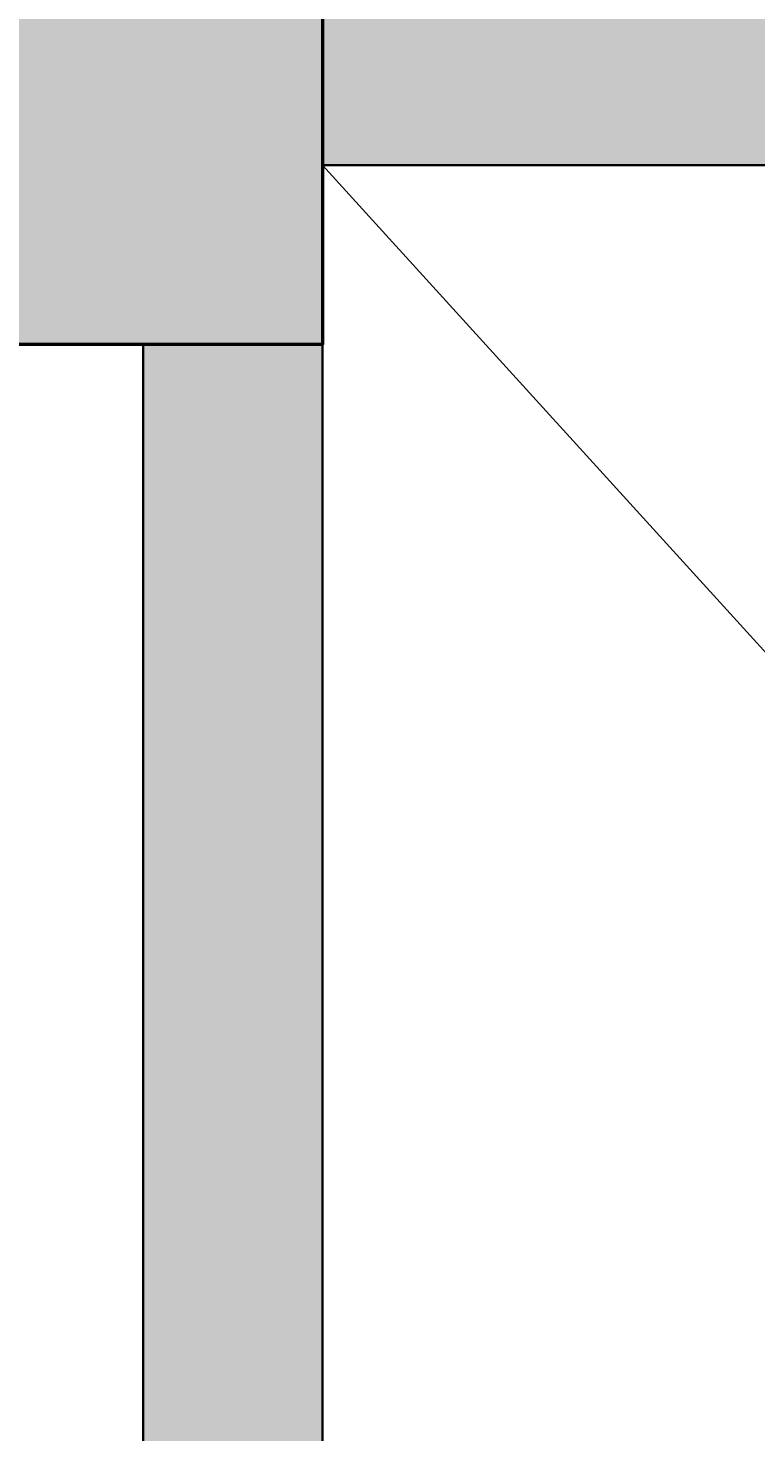
# Model space of a CAD drawing. Units: inches. Extents: x 1998 to 2588, y 1139 to 1977.
# Tile 33 of 134: x 2220 to 2238, y 1557 to 1592. Entities that reach past the tile are written whole.
import ezdxf

# ---------------------------------------------------------------- set-up
doc = ezdxf.new("R2010")
doc.units = ezdxf.units.IN
for name, color, linetype, lineweight in [('A-ANNO-DIMS', 2, 'Continuous', 18), ('A-COLS-PATT', 250, 'Continuous', 13), ('A-FLOR-OPEN', 8, 'Continuous', 18), ('A-WALL-PATT', 252, 'Continuous', 13), ('COLUMN', 10, 'Continuous', 50), ('WALL', 200, 'Continuous', 35)]:
    doc.layers.add(name, color=color, linetype=linetype, lineweight=lineweight)
doc.styles.get("Standard").update_dxf_attribs({"font": 'arial.ttf'})
doc.dimstyles.get("Standard").update_dxf_attribs({"dimtxt": 0.18, "dimasz": 0.18, "dimexe": 0.18, "dimexo": 0.0625, "dimgap": 0.09, "dimtad": 0, "dimtih": 1, "dimtoh": 1, "dimdec": 4, "dimzin": 0, "dimdsep": 46, "dimtxsty": 'Standard', "dimcen": 0.09, "dimadec": 0, "dimazin": 0, "dimtfac": 1, "dimtdec": 4, "dimtofl": 0, "dimtmove": 0, "dimatfit": 3, "dimfxl": 1, "dimtolj": 1, "dimtzin": 0, "dimarcsym": 0})

# ---------------------------------------------------------------- blocks, each defined once
blk = doc.blocks.new('*D34')
at = {"layer": 'A-ANNO-DIMS', "color": 0, "lineweight": -2, "transparency": 16777216}
for p, q in [((2407.91, 1594.732), (1997.843, 1594.732)), ((1998.023, 1594.552), (1998.023, 1558.913)), ((1998.023, 1522.912), (1998.023, 1558.552)), ((2407.91, 1522.732), (1997.843, 1522.732))]:
    blk.add_line(p, q, dxfattribs=at)
at = {"layer": 'A-ANNO-DIMS', "color": 0, "transparency": 16777216}
for points in [[(1997.993, 1594.552), (1998.053, 1594.552), (1998.023, 1594.732)], [(1997.993, 1522.912), (1998.053, 1522.912), (1998.023, 1522.732)]]:
    blk.add_solid(points, dxfattribs=at)
at = {"layer": 'Defpoints', "color": 0, "transparency": 16777216}
for p in [(1998.023, 1594.732), (2407.973, 1594.732), (2407.973, 1522.732)]:
    blk.add_point(p, dxfattribs=at)
at = {"layer": 'A-ANNO-DIMS', "color": 0, "transparency": 16777216, "insert": (1998.023, 1558.732), "char_height": 0.18, "attachment_point": 5}
blk.add_mtext('\\A1;72', dxfattribs=at)
blk = doc.blocks.new('*D41')
at = {"layer": 'A-ANNO-DIMS', "color": 0, "lineweight": -2, "transparency": 16777216}
for p, q in [((2227.473, 1588.67), (2227.473, 1138.602)), ((2287.473, 1588.67), (2287.473, 1138.602)), ((2227.653, 1138.782), (2257.254, 1138.782)), ((2287.293, 1138.782), (2257.692, 1138.782))]:
    blk.add_line(p, q, dxfattribs=at)
at = {"layer": 'A-ANNO-DIMS', "color": 0, "transparency": 16777216}
for points in [[(2227.653, 1138.812), (2227.653, 1138.752), (2227.473, 1138.782)], [(2287.293, 1138.812), (2287.293, 1138.752), (2287.473, 1138.782)]]:
    blk.add_solid(points, dxfattribs=at)
at = {"layer": 'Defpoints', "color": 0, "transparency": 16777216}
for p in [(2227.473, 1588.732), (2287.473, 1588.732), (2287.473, 1138.782)]:
    blk.add_point(p, dxfattribs=at)
at = {"layer": 'A-ANNO-DIMS', "color": 0, "transparency": 16777216, "insert": (2257.473, 1138.782), "char_height": 0.18, "attachment_point": 5}
blk.add_mtext('\\A1;60', dxfattribs=at)

msp = doc.modelspace()

# ---------------------------------------------------------------- hatches: boundary and pattern name
at = {"layer": 'A-COLS-PATT'}
h = msp.add_hatch(color=256, dxfattribs=at)
h.dxf.hatch_style = 1
h.paths.add_polyline_path([(2099.4125, 1888.7324), (2087.9729, 1888.7324), (2087.9729, 1868.3278), (2099.4125, 1868.3278)])
h.paths.add_polyline_path([(2234.4125, 1888.7324), (2222.9729, 1888.7324), (2222.9729, 1868.3278), (2234.4125, 1868.3278)])
h.paths.add_polyline_path([(2341.4729, 1886.637), (2330.0332, 1886.637), (2330.0332, 1866.2324), (2341.4729, 1866.2324)])
h.paths.add_polyline_path([(2507.8006, 1882.7324), (2487.396, 1882.7324), (2487.396, 1871.2927), (2507.8006, 1871.2927)])
h.paths.add_polyline_path([(2510.9729, 1766.672), (2490.5682, 1766.672), (2490.5682, 1755.2324), (2510.9729, 1755.2324)])
h.paths.add_polyline_path([(2345.9729, 1759.7324), (2334.5332, 1759.7324), (2334.5332, 1739.3278), (2345.9729, 1739.3278)])
h.paths.add_polyline_path([(2234.4125, 1774.3318), (2222.9729, 1774.3318), (2222.9729, 1753.9272), (2234.4125, 1753.9272)])
h.paths.add_polyline_path([(2099.4125, 1775.637), (2087.9729, 1775.637), (2087.9729, 1755.2324), (2099.4125, 1755.2324)])
h.paths.add_polyline_path([(2098.0956, 1593.7241), (2077.691, 1593.7241), (2077.691, 1582.2845), (2098.0956, 1582.2845)])
h.paths.add_polyline_path([(2227.4729, 1604.637), (2216.0332, 1604.637), (2216.0332, 1584.2324), (2227.4729, 1584.2324)])
h.paths.add_polyline_path([(2345.9729, 1647.5211), (2334.5332, 1647.5211), (2334.5332, 1627.1165), (2345.9729, 1627.1165)])
h.paths.add_polyline_path([(2522.3775, 1641.2324), (2501.9729, 1641.2324), (2501.9729, 1629.7927), (2522.3775, 1629.7927)])
h.paths.add_polyline_path([(2522.3775, 1480.7324), (2501.9729, 1480.7324), (2501.9729, 1469.2927), (2522.3775, 1469.2927)])
h.paths.add_polyline_path([(2345.9729, 1488.5616), (2334.5332, 1488.5616), (2334.5332, 1468.1569), (2345.9729, 1468.1569)])
h.paths.add_polyline_path([(2234.4125, 1486.137), (2227.4729, 1486.137), (2227.4729, 1465.7324), (2234.4125, 1465.7324)])
h.paths.add_polyline_path([(2227.4729, 1486.137), (2222.9729, 1486.137), (2222.9729, 1465.7324), (2227.4729, 1465.7324)])
h.paths.add_polyline_path([(2108.3775, 1470.2324), (2087.9729, 1470.2324), (2087.9729, 1458.7927), (2108.3775, 1458.7927)])
h.paths.add_polyline_path([(2096.9729, 1365.5012), (2087.9729, 1365.5012), (2087.9729, 1345.0966), (2096.9729, 1345.0966)])
h.paths.add_polyline_path([(2087.9729, 1365.5012), (2085.5332, 1365.5012), (2085.5332, 1345.0966), (2087.9729, 1345.0966)])
h.paths.add_polyline_path([(2234.4125, 1285.137), (2222.9729, 1285.137), (2222.9729, 1264.7324), (2234.4125, 1264.7324)])
h.paths.add_polyline_path([(2345.9729, 1285.137), (2334.5332, 1285.137), (2334.5332, 1264.7324), (2345.9729, 1264.7324)])
h.paths.add_polyline_path([(2503.1458, 1240.172), (2482.7412, 1240.172), (2482.7412, 1228.7324), (2503.1458, 1228.7324)])
h.paths.add_polyline_path([(2510.9729, 1369.172), (2490.5682, 1369.172), (2490.5682, 1357.7324), (2510.9729, 1357.7324)])
at = {"layer": 'A-WALL-PATT'}
h = msp.add_hatch(color=256, dxfattribs=at)
h.dxf.hatch_style = 1
h.paths.add_polyline_path([(2222.9729, 1888.7324), (2099.4125, 1888.7324), (2099.4125, 1879.7324), (2222.9729, 1879.7324)])
h.paths.add_polyline_path([(2096.9729, 1868.3278), (2087.9729, 1868.3278), (2087.9729, 1775.637), (2096.9729, 1775.637)])
h.paths.add_polyline_path([(2227.4729, 1868.3278), (2222.9729, 1868.3278), (2222.9729, 1774.3318), (2227.4729, 1774.3318)])
h.paths.add_polyline_path([(2188.3019, 1759.7324), (2138.6074, 1759.7324), (2099.4125, 1759.7324), (2099.4125, 1755.2324), (2176.9729, 1755.2324), (2188.3019, 1755.2324)])
h.paths.add_polyline_path([(2087.9729, 1759.7324), (2059.4729, 1759.7324), (2059.4729, 1702.7324), (2087.9729, 1702.7324), (2087.9729, 1707.2324), (2063.9729, 1707.2324), (2063.9729, 1755.2324), (2087.9729, 1755.2324)])
h.paths.add_polyline_path([(2096.9729, 1755.2324), (2087.9729, 1755.2324), (2087.9729, 1707.2324), (2096.9729, 1707.2324)])
h.paths.add_polyline_path([(2187.0461, 1707.2324), (2105.9729, 1707.2324), (2096.9729, 1707.2324), (2087.9729, 1707.2324), (2087.9729, 1702.7324), (2105.9729, 1702.7324), (2114.9729, 1702.7324), (2187.0461, 1702.7324)])
h.paths.add_polyline_path([(2181.4729, 1719.2028), (2176.9729, 1719.2028), (2176.9729, 1707.2324), (2181.4729, 1707.2324)])
h.paths.add_polyline_path([(2216.0332, 1588.7324), (2114.9729, 1588.7324), (2105.9729, 1588.7324), (2105.9729, 1584.2324), (2216.0332, 1584.2324)])
h.paths.add_polyline_path([(2077.691, 1588.7324), (2061.4729, 1588.7324), (2061.4729, 1584.2324), (2077.691, 1584.2324)])
h.paths.add_polyline_path([(2105.9729, 1588.7324), (2098.0956, 1588.7324), (2098.0956, 1584.2324), (2105.9729, 1584.2324)])
h.paths.add_polyline_path([(2114.9729, 1596.2642), (2110.1012, 1596.2642), (2105.9729, 1596.2642), (2105.9729, 1588.7324), (2114.9729, 1588.7324)])
h.paths.add_polyline_path([(2114.9729, 1584.2324), (2105.9729, 1584.2324), (2105.9729, 1580.249), (2110.1012, 1580.249), (2114.9729, 1580.249)])
h.paths.add_polyline_path([(2114.9729, 1547.7716), (2110.1012, 1547.7716, -0.0318759), (2105.9729, 1548.035), (2105.9729, 1470.2324), (2108.3775, 1470.2324), (2108.3775, 1465.7324), (2186.2943, 1465.7324), (2186.2943, 1470.2324), (2114.9729, 1470.2324)])
h.paths.add_polyline_path([(2227.4729, 1584.2324), (2222.9729, 1584.2324), (2222.9729, 1486.137), (2227.4729, 1486.137)])
h.paths.add_polyline_path([(2295.4138, 1593.2324), (2227.4729, 1593.2324), (2227.4729, 1588.7324), (2295.4138, 1588.7324), (2295.4138, 1591.8729)])
h.paths.add_polyline_path([(2345.9729, 1627.1165), (2341.4729, 1627.1165), (2341.4729, 1593.2324), (2337.2869, 1593.2324), (2337.2869, 1591.8729), (2337.2869, 1588.7324), (2345.9729, 1588.7324)])
h.paths.add_polyline_path([(2291.9729, 1588.7324), (2287.4729, 1588.7324), (2287.4729, 1522.7324), (2291.9729, 1522.7324)])
h.paths.add_polyline_path([(2291.9729, 1522.7324), (2287.4729, 1522.7324), (2227.4729, 1522.7324), (2227.4729, 1518.2324), (2291.9729, 1518.2324)])
h.paths.add_polyline_path([(2295.7347, 1519.5919), (2295.7347, 1522.7324), (2291.9729, 1522.7324), (2291.9729, 1518.2324), (2295.7347, 1518.2324)])
h.paths.add_polyline_path([(2345.9729, 1522.7324), (2337.6078, 1522.7324), (2337.6078, 1519.5919), (2337.6078, 1518.2324), (2341.4729, 1518.2324), (2341.4729, 1488.5616), (2345.9729, 1488.5616)])
h.paths.add_polyline_path([(2345.9729, 1468.1569), (2341.4729, 1468.1569), (2341.4729, 1374.2324), (2227.4729, 1374.2324), (2227.4729, 1369.7324), (2345.9729, 1369.7324)])
h.paths.add_polyline_path([(2345.9729, 1369.7324), (2341.4729, 1369.7324), (2341.4729, 1362.2324), (2345.9729, 1362.2324)])
h.paths.add_polyline_path([(2345.9729, 1317.7324), (2345.9729, 1322.2324), (2341.4729, 1322.2324), (2341.4729, 1285.137), (2345.9729, 1285.137)], flags=17)
h.paths.add_polyline_path([(2356.2096, 1322.2324), (2345.9729, 1322.2324), (2345.9729, 1317.7324), (2356.2096, 1317.7324), (2356.2096, 1319.3088)], flags=17)
h.paths.add_polyline_path([(2393.9729, 1322.2324), (2375.6999, 1322.2324), (2375.6999, 1319.3088, -0.0202458), (2375.636, 1317.7324), (2393.9729, 1317.7324)], flags=17)
h.paths.add_polyline_path([(2398.4729, 1322.2324), (2393.9729, 1322.2324), (2393.9729, 1317.7324), (2393.9729, 1237.7324), (2345.9729, 1237.7324), (2345.9729, 1264.7324), (2341.4729, 1264.7324), (2341.4729, 1228.7324), (2393.9729, 1228.7324), (2482.7412, 1228.7324), (2482.7412, 1237.7324), (2398.4729, 1237.7324), (2398.4729, 1297.1029)])
h.paths.add_polyline_path([(2398.4729, 1362.2324), (2393.9729, 1362.2324), (2393.9729, 1357.7324), (2398.4729, 1357.7324)])
h.paths.add_polyline_path([(2345.9729, 1329.7549), (2341.4729, 1329.7549), (2341.4729, 1322.2324), (2345.9729, 1322.2324)])

# ---------------------------------------------------------------- linework, layer by layer
at = {"layer": 'A-FLOR-OPEN'}
msp.add_line((2227.4729, 1588.7324), (2287.4729, 1522.7324), dxfattribs=at)
at = {"layer": 'COLUMN'}
msp.add_lwpolyline([(2216.0332, 1604.637), (2227.4729, 1604.637), (2227.4729, 1584.2324), (2216.0332, 1584.2324)], close=True, dxfattribs=at)
at = {"layer": 'WALL'}
for p, q in [((2227.4729, 1707.2324), (2227.4729, 1584.2324)), ((2227.4729, 1588.7324), (2227.4729, 1486.137)), ((2227.4729, 1588.7324), (2227.4729, 1522.7324)), ((2295.4138, 1588.7324), (2227.4729, 1588.7324)), ((2227.4729, 1584.2324), (2105.9729, 1584.2324)), ((2222.9729, 1584.2324), (2222.9729, 1486.137))]:
    msp.add_line(p, q, dxfattribs=at)

# ---------------------------------------------------------------- dimensions: what is measured, and where the dimension line sits
at = {"layer": 'A-ANNO-DIMS'}
dim = msp.add_linear_dim(base=(1998.0229, 1594.7324), p1=(2407.9729, 1522.7324), p2=(2407.9729, 1594.7324), angle=90, dimstyle='Standard', override={"dimdec": 0, "dimlfac": 1, "dimrnd": 0, "dimzin": 0, "dimdsep": 46, "dimlunit": 2}, dxfattribs=at)
dim.commit()
dim.dimension.update_dxf_attribs({"geometry": '*D34', "text_midpoint": (1998.0229, 1558.7324)})
dim = msp.add_linear_dim(base=(2287.4729, 1138.7824), p1=(2227.4729, 1588.7324), p2=(2287.4729, 1588.7324), dimstyle='Standard', override={"dimdec": 0, "dimlfac": 1, "dimrnd": 0, "dimzin": 0, "dimdsep": 46, "dimlunit": 2}, dxfattribs=at)
dim.commit()
dim.dimension.update_dxf_attribs({"geometry": '*D41', "text_midpoint": (2257.4729, 1138.7824)})

doc.saveas('drawing.dxf')
